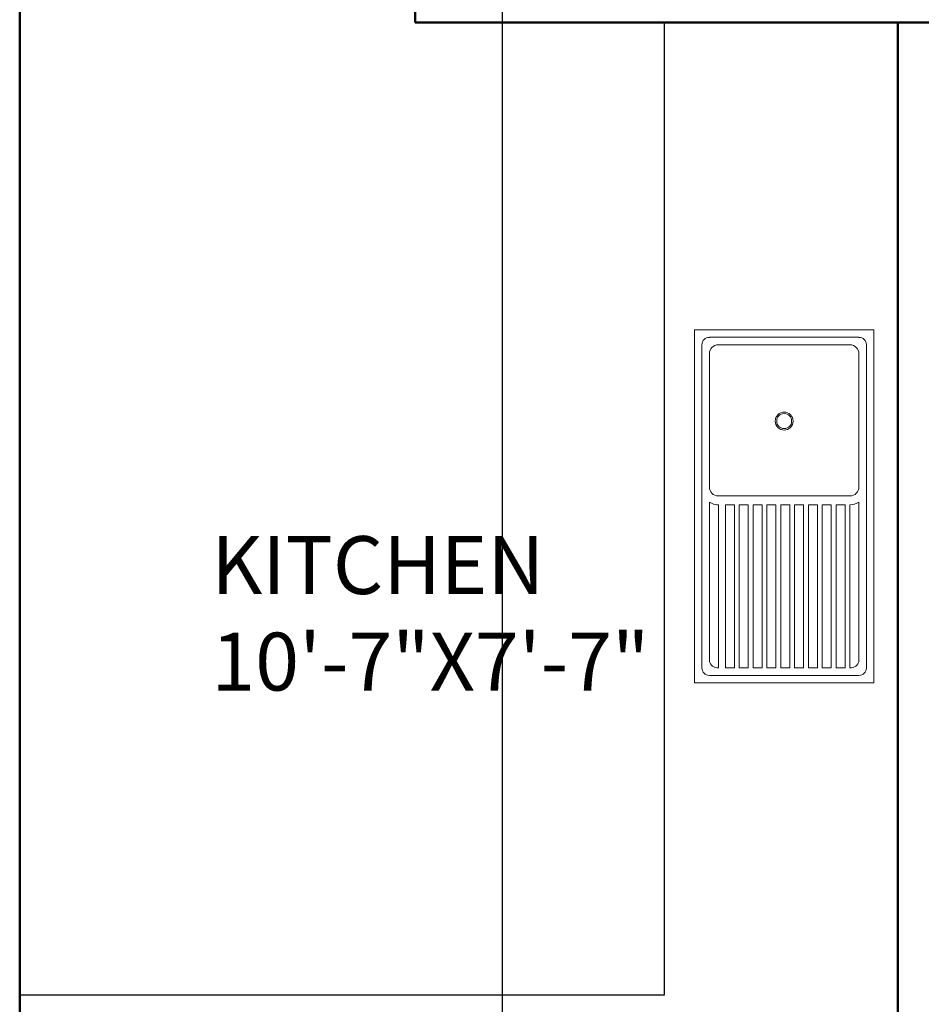
# Model space of a CAD drawing. Units: inches. Extents: x -173 to 545, y -746 to 104.
# Tile 7 of 32: x 170 to 263, y -663 to -561. Entities that reach past the tile are written whole.
import ezdxf

# ---------------------------------------------------------------- set-up
doc = ezdxf.new("R2010")
doc.units = ezdxf.units.IN
doc.header["$MEASUREMENT"] = 0
for name, color, linetype, lineweight in [('A-ANNO-DIMS', 2, 'Continuous', 18), ('A-AREA-IDEN', 7, 'Continuous', 18), ('A-FLOR-CASE', 9, 'Continuous', 25), ('A-FLOR-FIXT', 8, 'Continuous', 18), ('A-WALL', 7, 'Continuous', 50)]:
    doc.layers.add(name, color=color, linetype=linetype, lineweight=lineweight)
doc.styles.get("Standard").update_dxf_attribs({"font": 'arial.ttf'})
doc.dimstyles.get("Standard").update_dxf_attribs({"dimtxt": 0.18, "dimasz": 0.18, "dimexe": 0.18, "dimexo": 0.0625, "dimgap": 0.09, "dimtad": 0, "dimtih": 1, "dimtoh": 1, "dimdec": 0, "dimzin": 0, "dimdsep": 46, "dimlunit": 3, "dimtxsty": 'Standard', "dimcen": 0.09, "dimadec": 0, "dimazin": 0, "dimtfac": 1, "dimtdec": 0, "dimtofl": 0, "dimtmove": 0, "dimatfit": 3, "dimfxl": 1, "dimtolj": 1, "dimtzin": 0, "dimarcsym": 0})

# ---------------------------------------------------------------- blocks, each defined once
blk = doc.blocks.new('М11 540х1060')
for p, q in [((-1062, 540), (0, 540)), ((-1062, 0), (-1062, 540)), ((0, 540), (0, 0)), ((-1017, 517.5), (-45, 517.5)), ((-1039.5, 45), (-1039.5, 495)), ((-990, 495), (-589.5, 495)), ((-543.7, 495), (-64.8, 495)), ((-22.5, 495), (-22.5, 45)), ((-1017, 72), (-1017, 468)), ((-562.5, 72), (-562.5, 468)), ((-535.7, 468), (-45, 468)), ((-535.7, 453.4), (-45, 453.4)), ((-535.7, 453.4), (-535.7, 426.4)), ((-45, 469.5), (-45, 468)), ((-45, 453.4), (-45, 426.4)), ((-535.7, 426.4), (-45, 426.4)), ((-535.7, 411.8), (-535.7, 384.8)), ((-535.7, 411.8), (-45, 411.8)), ((-45, 411.8), (-45, 384.8)), ((-535.7, 384.8), (-45, 384.8)), ((-535.7, 370.1), (-535.7, 343.1)), ((-535.7, 370.1), (-45, 370.1)), ((-45, 370.1), (-45, 343.1)), ((-535.7, 343.1), (-45, 343.1)), ((-535.7, 328.5), (-535.7, 301.5)), ((-535.7, 328.5), (-45, 328.5)), ((-45, 328.5), (-45, 301.5)), ((-535.7, 301.5), (-45, 301.5)), ((-535.7, 286.9), (-535.7, 259.9)), ((-535.7, 286.9), (-45, 286.9)), ((-45, 286.9), (-45, 259.9)), ((-535.7, 259.9), (-45, 259.9)), ((-535.7, 245.3), (-535.7, 218.3)), ((-535.7, 245.3), (-45, 245.3)), ((-45, 245.3), (-45, 218.3)), ((-535.7, 218.3), (-45, 218.3)), ((-535.7, 203.6), (-535.7, 176.6)), ((-535.7, 203.6), (-45, 203.6)), ((-45, 203.6), (-45, 176.6)), ((-535.7, 176.6), (-45, 176.6)), ((-535.7, 162), (-45, 162)), ((-535.7, 162), (-535.7, 135)), ((-45, 162), (-45, 135)), ((-535.7, 135), (-45, 135)), ((-535.7, 120.4), (-45, 120.4)), ((-535.7, 120.4), (-535.7, 93.4)), ((-45, 120.4), (-45, 93.4)), ((-535.7, 93.4), (-45, 93.4)), ((-535.7, 72), (-45, 72)), ((-535.7, 72), (-535.7, 67.5)), ((-45, 70.5), (-45, 72)), ((-589.5, 45), (-990, 45)), ((-543.7, 45), (-64.8, 45)), ((0, 0), (-1062, 0)), ((-45, 22.5), (-1017, 22.5))]:
    blk.add_line(p, q)
for centre, major_axis, start_param, end_param in [((-1017, 495), (-15.9, 15.9), -0.785398, 0.785398), ((-45, 495), (15.9, 15.9), 5.497787, 7.068583), ((-990, 468), (19.1, 19.1), 0.785398, 2.356194), ((-589.5, 468), (-19.1, 19.1), 3.926991, 5.497787), ((-585.2, 468), (-35, 35), 3.926991, 4.503922), ((-72.3, 468.8), (-19.3, 19.3), 3.899365, 5.250385), ((-787.5, 270), (-19.1, 19.1), 3.926991, 10.210176), ((-787.5, 270), (-15.9, 15.9), 3.926991, 10.210176), ((-990, 72), (-19.1, 19.1), 0.785398, 2.356194), ((-589.5, 72), (19.1, 19.1), 3.926991, 5.497787), ((-585.2, 72), (35, 35), 4.920856, 5.497787), ((-72.3, 71.2), (19.3, 19.3), 4.174393, 5.525413), ((-1017, 45), (15.9, 15.9), 2.356194, 3.926991), ((-45, 45), (-15.9, 15.9), 2.356194, 3.926991)]:
    blk.add_ellipse(centre, major_axis=major_axis, ratio=1, start_param=start_param, end_param=end_param)
blk = doc.blocks.new('*D81')
at = {"layer": 'A-ANNO-DIMS', "color": 0, "lineweight": -2, "transparency": 16777216}
for p, q in [((219.8, -551.92), (219.8, -740.64)), ((306.3, -551.92), (306.3, -740.64)), ((219.98, -740.46), (262.51, -740.46)), ((306.12, -740.46), (263.59, -740.46))]:
    blk.add_line(p, q, dxfattribs=at)
at = {"layer": 'A-ANNO-DIMS', "color": 0, "transparency": 16777216}
for points in [[(219.98, -740.43), (219.98, -740.49), (219.8, -740.46)], [(306.12, -740.43), (306.12, -740.49), (306.3, -740.46)]]:
    blk.add_solid(points, dxfattribs=at)
at = {"layer": 'Defpoints', "color": 0, "transparency": 16777216}
for p in [(219.8, -551.86), (306.3, -551.86), (306.3, -740.46)]:
    blk.add_point(p, dxfattribs=at)
at = {"layer": 'A-ANNO-DIMS', "color": 0, "transparency": 16777216, "insert": (263.05, -740.46), "char_height": 0.18, "attachment_point": 5}
blk.add_mtext('\\A1;7\'-2 1/2"', dxfattribs=at)

msp = doc.modelspace()

# ---------------------------------------------------------------- linework, layer by layer
at = {"layer": 'A-FLOR-CASE'}
for p, q in [((236.59, -560.86), (236.59, -661.64)), ((236.59, -661.64), (169.8, -661.64))]:
    msp.add_line(p, q, dxfattribs=at)
at = {"layer": 'A-WALL'}
for p, q in [((210.8, -463.36), (210.8, -560.86)), ((169.8, -551.86), (169.8, -688.36)), ((210.8, -560.86), (315.3, -560.86)), ((260.8, -560.86), (260.8, -688.36))]:
    msp.add_line(p, q, dxfattribs=at)

# ---------------------------------------------------------------- block references
at = {"layer": 'A-FLOR-FIXT', "xscale": 0.0344518369672997, "yscale": 0.0344518369672997, "zscale": 0.0344518369672997, "rotation": 270}
msp.add_blockref('М11 540х1060', (239.73, -629.29), dxfattribs=at)

# ---------------------------------------------------------------- texts
at = {"layer": 'A-AREA-IDEN', "insert": (189.67, -614.08), "char_height": 6, "attachment_point": 1}
msp.add_mtext('KITCHEN\\P10\'-7"X7\'-7"', dxfattribs=at)

# ---------------------------------------------------------------- dimensions: what is measured, and where the dimension line sits
at = {"layer": 'A-ANNO-DIMS'}
dim = msp.add_linear_dim(base=(306.3, -740.46), p1=(219.8, -551.86), p2=(306.3, -551.86), dimstyle='Standard', override={"dimdec": 1, "dimlfac": 1, "dimrnd": 0, "dimzin": 1, "dimdsep": 46, "dimlunit": 4, "dimfrac": 2}, dxfattribs=at)
dim.commit()
dim.dimension.update_dxf_attribs({"geometry": '*D81', "text_midpoint": (263.05, -740.46)})

doc.saveas('drawing.dxf')
